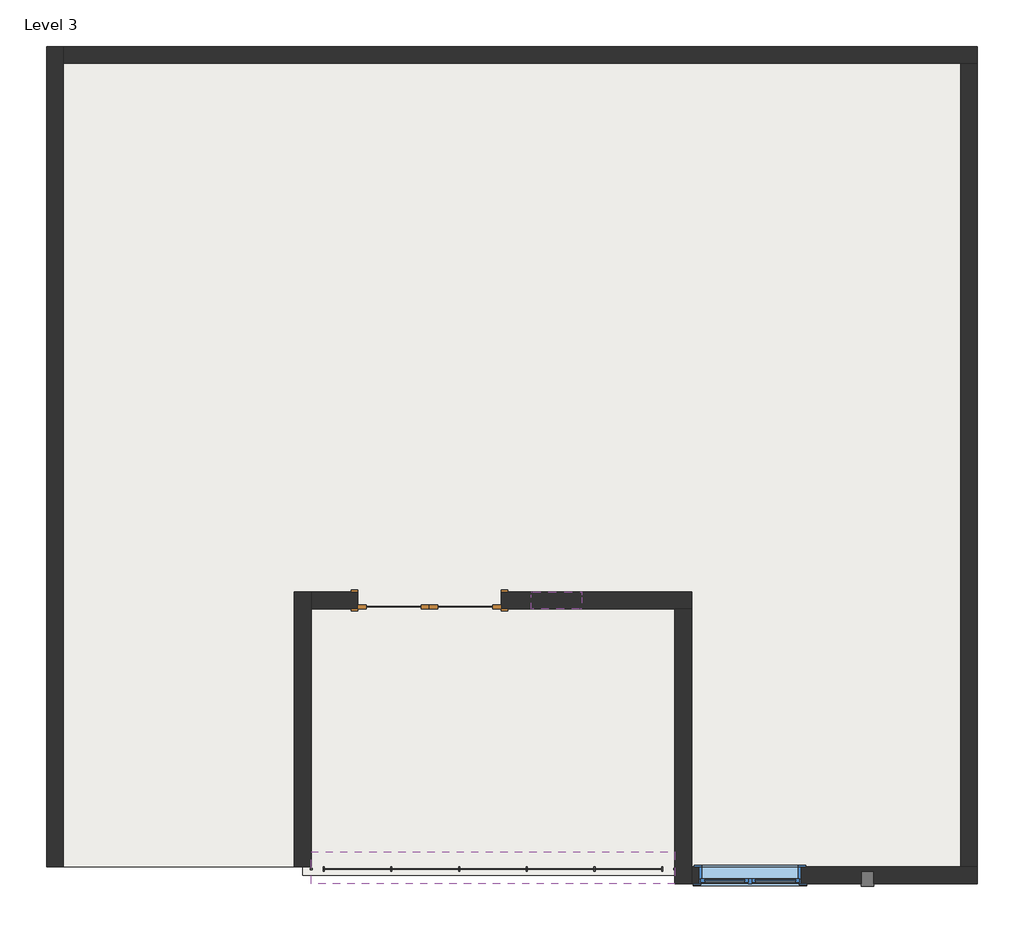
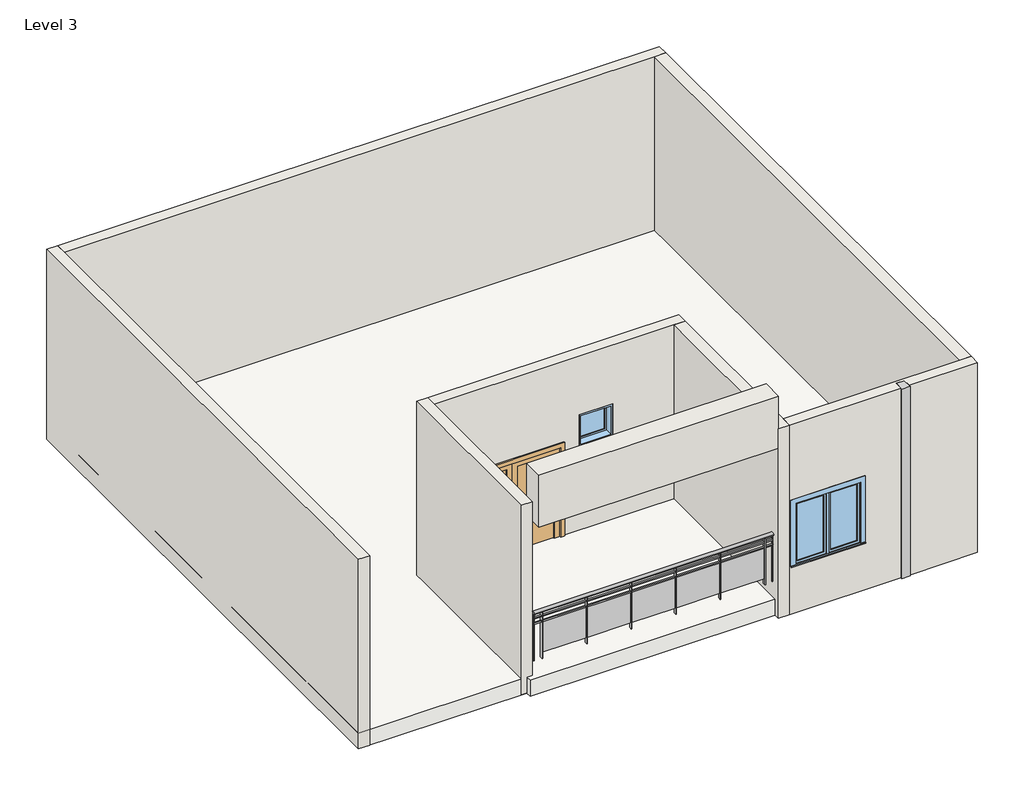
# One storey: 8 walls, 2 windows, 1 door, 1 proxy, 1 railing, 1 roof.
"""IFC4 building model written with IfcOpenShell, lengths in millimetres."""

from ifc_helpers import new_model, si_unit, point, frame, origin, place, context, project, spatial, polyline, ellipse_curve, trimmed, outline, extrude, faceted_brep, transform, mapped, element, save
from ifc_brep_helpers import plane_surface, extruded_surface, advanced_brep
from components import door_10418eaf, walls_2_walls_2_a0716ef0, window_0862ab64, window_6846e476

model = new_model("IFC4")

# Units and contexts
model_context = context("Model", 3, world=origin())
ifc_project = project(units=[si_unit("LENGTHUNIT", "METRE", prefix="MILLI")], contexts=[model_context])

# Site, building, storey
site = spatial("IfcSite", under=ifc_project)
building = spatial("IfcBuilding", under=site)
storey = spatial("IfcBuildingStorey", under=building, Name="Level 3", Elevation=7315.2)

# Proxy
placement = place(None, origin())
element("IfcBuildingElementProxy", 1, Name="Reveal", ObjectType="Reveal", at=placement, inside=storey, context=model_context, shape_type="SweptSolid", body=[
    extrude(outline(polyline([(752.5001186, 242.2810824), (752.5001186, 425.1610824), (904.9001186, 425.1610824), (904.9001186, 242.2810824), (752.5001186, 242.2810824)])), frame((0.0, 0.0, 7315.2), z_axis=(0.0, 0.0, 1.0), x_axis=(1.0, 0.0, 0.0)), (0.0, 0.0, 1.0), 3657.6),
])

# Door
door_shape = door_10418eaf(model_context)
element("IfcDoor", 2, ObjectType="Door-Double-Glass : 68\" x 80\"", at=placement, inside=storey, context=model_context, shape_type="MappedRepresentation", body=[
    mapped(door_shape, transform((-4429.0998814, 3678.7423324, 7315.2), x_axis=(-1.0, 0.0, 0.0), y_axis=(0.0, -1.0, 0.0), z_axis=(0.0, 0.0, 1.0))),
])

# Railing
element("IfcRailing", 3, ObjectType="Glass Panel - Bottom Fill", at=placement, inside=storey, context=model_context, shape_type="SolidModel", body=[
    advanced_brep(
    [(-5851.4998814, 488.6610824, 8839.2), (-5851.4998814, 412.4610824, 8839.2), (-1482.6998814, 488.6610824, 8839.2), (-1482.6998814, 412.4610824, 8839.2)],
    [
        (0, 1, ellipse_curve(frame((-5851.4998814, 450.5610824, 8839.2), z_axis=(-1.0, 0.0, 0.0), x_axis=(0.0, -1.0, 0.0)), 38.1, 28.575)),
        (1, 0, ellipse_curve(frame((-5851.4998814, 450.5610824, 8839.2), z_axis=(-1.0, 0.0, 0.0), x_axis=(0.0, -1.0, 0.0)), 38.1, 28.575)),
        (2, 3, ellipse_curve(frame((-1482.6998814, 450.5610824, 8839.2), z_axis=(1.0, 0.0, 0.0), x_axis=(0.0, -1.0, 0.0)), 38.1, 28.575)),
        (3, 2, ellipse_curve(frame((-1482.6998814, 450.5610824, 8839.2), z_axis=(1.0, 0.0, 0.0), x_axis=(0.0, -1.0, 0.0)), 38.1, 28.575)),
        (0, 2),
        (3, 1),
    ],
    [
        plane_surface(frame((-5851.4998814, 450.5610824, 8839.2), z_axis=(-1.0, 0.0, 0.0), x_axis=(0.0, 1.0, 0.0))),
        plane_surface(frame((-1482.6998814, 450.5610824, 8839.2), z_axis=(1.0, 0.0, 0.0), x_axis=(0.0, 1.0, 0.0))),
        extruded_surface(trimmed(ellipse_curve(frame((-1482.6998814, 450.5610824, 8839.2), z_axis=(-1.0, 0.0, 0.0), x_axis=(0.0, -1.0, 0.0)), 38.1, 28.575), [point((-1482.6998814, 488.6610824, 8839.2))], [point((-1482.6998814, 412.4610824, 8839.2))], True, "CARTESIAN"), (-4368.8, 0.0, 0.0), 4368.8),
        extruded_surface(trimmed(ellipse_curve(frame((-1482.6998814, 450.5610824, 8839.2), z_axis=(-1.0, 0.0, 0.0), x_axis=(0.0, -1.0, 0.0)), 38.1, 28.575), [point((-1482.6998814, 412.4610824, 8839.2))], [point((-1482.6998814, 488.6610824, 8839.2))], True, "CARTESIAN"), (-4368.8, 0.0, 0.0), 4368.8),
    ],
    [
        (0, [[1, 2]]),
        (1, [[3, 4]]),
        (2, [[-1, 5, -4, 6]]),
        (3, [[-2, -6, -3, -5]]),
    ],
),
    extrude(outline(polyline([(-5851.4998814, 437.8610824), (-5851.4998814, 463.2610824), (-1482.6998814, 463.2610824), (-1482.6998814, 437.8610824), (-5851.4998814, 437.8610824)])), frame((0.0, 0.0, 8724.9), z_axis=(0.0, 0.0, 1.0), x_axis=(1.0, 0.0, 0.0)), (0.0, 0.0, 1.0), 25.4),
    extrude(outline(polyline([(-5851.4998814, 437.8610824), (-5851.4998814, 463.2610824), (-1482.6998814, 463.2610824), (-1482.6998814, 437.8610824), (-5851.4998814, 437.8610824)])), frame((0.0, 0.0, 8623.3), z_axis=(0.0, 0.0, 1.0), x_axis=(1.0, 0.0, 0.0)), (0.0, 0.0, 1.0), 25.4),
    extrude(outline(polyline([(-1641.4498814, 425.1610824), (-1641.4498814, 475.9610824), (-1628.7498814, 475.9610824), (-1628.7498814, 425.1610824), (-1641.4498814, 425.1610824)])), frame((0.0, 0.0, 7924.8), z_axis=(0.0, 0.0, 1.0), x_axis=(1.0, 0.0, 0.0)), (0.0, 0.0, 1.0), 885.6788223),
    extrude(outline(polyline([(-2447.8998814, 457.0962394), (-1635.0998814, 457.0962394), (-1635.0998814, 450.7462394), (-2447.8998814, 450.7462394), (-2447.8998814, 457.0962394)])), frame((0.0, 0.0, 8026.4), z_axis=(0.0, 0.0, 1.0), x_axis=(1.0, 0.0, 0.0)), (0.0, 0.0, 1.0), 596.9),
    extrude(outline(polyline([(-2454.2498814, 425.1610824), (-2454.2498814, 475.9610824), (-2441.5498814, 475.9610824), (-2441.5498814, 425.1610824), (-2454.2498814, 425.1610824)])), frame((0.0, 0.0, 7924.8), z_axis=(0.0, 0.0, 1.0), x_axis=(1.0, 0.0, 0.0)), (0.0, 0.0, 1.0), 885.6788223),
    extrude(outline(polyline([(-3260.6998814, 457.0962394), (-2447.8998814, 457.0962394), (-2447.8998814, 450.7462394), (-3260.6998814, 450.7462394), (-3260.6998814, 457.0962394)])), frame((0.0, 0.0, 8026.4), z_axis=(0.0, 0.0, 1.0), x_axis=(1.0, 0.0, 0.0)), (0.0, 0.0, 1.0), 596.9),
    extrude(outline(polyline([(-3267.0498814, 425.1610824), (-3267.0498814, 475.9610824), (-3254.3498814, 475.9610824), (-3254.3498814, 425.1610824), (-3267.0498814, 425.1610824)])), frame((0.0, 0.0, 7924.8), z_axis=(0.0, 0.0, 1.0), x_axis=(1.0, 0.0, 0.0)), (0.0, 0.0, 1.0), 885.6788223),
    extrude(outline(polyline([(-4073.4998814, 457.0962394), (-3260.6998814, 457.0962394), (-3260.6998814, 450.7462394), (-4073.4998814, 450.7462394), (-4073.4998814, 457.0962394)])), frame((0.0, 0.0, 8026.4), z_axis=(0.0, 0.0, 1.0), x_axis=(1.0, 0.0, 0.0)), (0.0, 0.0, 1.0), 596.9),
    extrude(outline(polyline([(-4079.8498814, 425.1610824), (-4079.8498814, 475.9610824), (-4067.1498814, 475.9610824), (-4067.1498814, 425.1610824), (-4079.8498814, 425.1610824)])), frame((0.0, 0.0, 7924.8), z_axis=(0.0, 0.0, 1.0), x_axis=(1.0, 0.0, 0.0)), (0.0, 0.0, 1.0), 885.6788223),
    extrude(outline(polyline([(-4886.2998814, 457.0962394), (-4073.4998814, 457.0962394), (-4073.4998814, 450.7462394), (-4886.2998814, 450.7462394), (-4886.2998814, 457.0962394)])), frame((0.0, 0.0, 8026.4), z_axis=(0.0, 0.0, 1.0), x_axis=(1.0, 0.0, 0.0)), (0.0, 0.0, 1.0), 596.9),
    extrude(outline(polyline([(-4892.6498814, 425.1610824), (-4892.6498814, 475.9610824), (-4879.9498814, 475.9610824), (-4879.9498814, 425.1610824), (-4892.6498814, 425.1610824)])), frame((0.0, 0.0, 7924.8), z_axis=(0.0, 0.0, 1.0), x_axis=(1.0, 0.0, 0.0)), (0.0, 0.0, 1.0), 885.6788223),
    extrude(outline(polyline([(-5699.0998814, 457.0962394), (-4886.2998814, 457.0962394), (-4886.2998814, 450.7462394), (-5699.0998814, 450.7462394), (-5699.0998814, 457.0962394)])), frame((0.0, 0.0, 8026.4), z_axis=(0.0, 0.0, 1.0), x_axis=(1.0, 0.0, 0.0)), (0.0, 0.0, 1.0), 596.9),
    extrude(outline(polyline([(-5705.4498814, 425.1610824), (-5705.4498814, 475.9610824), (-5692.7498814, 475.9610824), (-5692.7498814, 425.1610824), (-5705.4498814, 425.1610824)])), frame((0.0, 0.0, 7924.8), z_axis=(0.0, 0.0, 1.0), x_axis=(1.0, 0.0, 0.0)), (0.0, 0.0, 1.0), 885.6788223),
    extrude(outline(polyline([(-1495.3998814, 441.0360824), (-1495.3998814, 460.0860824), (-1476.3498814, 460.0860824), (-1476.3498814, 441.0360824), (-1495.3998814, 441.0360824)])), frame((0.0, 0.0, 7924.8), z_axis=(0.0, 0.0, 1.0), x_axis=(1.0, 0.0, 0.0)), (0.0, 0.0, 1.0), 885.6788223),
    extrude(outline(polyline([(-5857.8498814, 441.0360824), (-5857.8498814, 460.0860824), (-5838.7998814, 460.0860824), (-5838.7998814, 441.0360824), (-5857.8498814, 441.0360824)])), frame((0.0, 0.0, 7924.8), z_axis=(0.0, 0.0, 1.0), x_axis=(1.0, 0.0, 0.0)), (0.0, 0.0, 1.0), 885.6788223),
])

# Roof
element("IfcRoof", 4, ObjectType="Generic - 12\"", at=placement, inside=storey, context=model_context, shape_type="SweptSolid", body=[
    extrude(outline(polyline([(-9026.4998814, 10331.1610824), (2149.5001186, 10331.1610824), (2149.5001186, 374.3610824), (-5953.0998814, 374.3610824), (-5953.0998814, 475.9610824), (-9026.4998814, 475.9610824), (-9026.4998814, 10331.1610824)])), frame((0.0, 0.0, 7315.2), z_axis=(0.0, 0.0, 1.0), x_axis=(1.0, 0.0, 0.0)), (0.0, 0.0, 1.0), 304.8),
])

# Walls
element("IfcWall", 5, ObjectType="Generic - 8\"", at=placement, inside=storey, context=model_context, shape_type="Brep", body=[
    faceted_brep([(-5851.4998814, 475.9610824, 7315.2), (-5851.4998814, 3574.7610824, 7315.2), (-5851.4998814, 3777.9610824, 7315.2), (-5851.4998814, 3777.9610824, 10972.8), (-5851.4998814, 3574.7610824, 10972.8), (-5851.4998814, 475.9610824, 10972.8), (-6054.6998814, 475.9610824, 7315.2), (-6054.6998814, 475.9610824, 10972.8), (-6054.6998814, 3777.9610824, 10972.8), (-6054.6998814, 3777.9610824, 7315.2)], [[[0, 1, 2, 3, 4, 5]], [[6, 7, 8, 9]], [[2, 1, 0, 6, 9]], [[5, 4, 3, 8, 7]], [[0, 5, 7, 6]], [[3, 2, 9, 8]]]),
])
element("IfcWall", 6, ObjectType="Generic - 8\"", at=placement, inside=storey, context=model_context, shape_type="Brep", body=[
    faceted_brep([(-5851.4998814, 3574.7610824, 7315.2), (-5292.6998814, 3574.7610824, 7315.2), (-5292.6998814, 3574.7610824, 9347.2), (-3565.4998814, 3574.7610824, 9347.2), (-3565.4998814, 3574.7610824, 7315.2), (-1482.6998814, 3574.7610824, 7315.2), (-1279.4998814, 3574.7610824, 7315.2), (-1279.4998814, 3574.7610824, 10972.8), (-1482.6998814, 3574.7610824, 10972.8), (-5851.4998814, 3574.7610824, 10972.8), (-2600.2998814, 3574.7610824, 9842.1899962), (-2600.2998814, 3574.7610824, 9232.5899962), (-3209.8998814, 3574.7610824, 9232.5899962), (-3209.8998814, 3574.7610824, 9842.1899962), (-5292.6998814, 3777.9610824, 9347.2), (-5292.6998814, 3777.9610824, 7315.2), (-5851.4998814, 3777.9610824, 7315.2), (-5851.4998814, 3777.9610824, 10972.8), (-1279.4998814, 3777.9610824, 10972.8), (-1279.4998814, 3777.9610824, 7315.2), (-3565.4998814, 3777.9610824, 7315.2), (-3565.4998814, 3777.9610824, 9347.2), (-2600.2998814, 3777.9610824, 9842.1899962), (-3209.8998814, 3777.9610824, 9842.1899962), (-3209.8998814, 3777.9610824, 9232.5899962), (-2600.2998814, 3777.9610824, 9232.5899962)], [[[0, 1, 2, 3, 4, 5, 6, 7, 8, 9], [10, 11, 12, 13]], [[14, 15, 16, 17, 18, 19, 20, 21], [22, 23, 24, 25]], [[20, 19, 6, 5, 4]], [[16, 15, 1, 0]], [[9, 8, 7, 18, 17]], [[0, 9, 17, 16]], [[7, 6, 19, 18]], [[11, 10, 22, 25]], [[12, 11, 25, 24]], [[13, 12, 24, 23]], [[10, 13, 23, 22]], [[2, 1, 15, 14]], [[3, 2, 14, 21]], [[4, 3, 21, 20]]]),
])
element("IfcWall", 7, ObjectType="Generic - 8\"", at=placement, inside=storey, context=model_context, shape_type="Brep", body=[
    faceted_brep([(-1482.6998814, 3574.7610824, 7315.2), (-1482.6998814, 272.7610824, 7315.2), (-1482.6998814, 272.7610824, 10972.8), (-1482.6998814, 3574.7610824, 10972.8), (-1279.4998814, 3574.7610824, 7315.2), (-1279.4998814, 3574.7610824, 10972.8), (-1279.4998814, 475.9610824, 10972.8), (-1279.4998814, 272.7610824, 10972.8), (-1279.4998814, 272.7610824, 7315.2), (-1279.4998814, 475.9610824, 7315.2)], [[[0, 1, 2, 3]], [[4, 5, 6, 7, 8, 9]], [[1, 0, 4, 9, 8]], [[3, 2, 7, 6, 5]], [[0, 3, 5, 4]], [[2, 1, 8, 7]]]),
])
element("IfcWall", 8, ObjectType="Generic - 8\"", at=placement, inside=storey, context=model_context, shape_type="Brep", body=[
    faceted_brep([(-1279.4998814, 272.7610824, 10972.8), (-1279.4998814, 272.7610824, 7315.2), (752.5001186, 272.7610824, 7315.2), (752.5001186, 272.7610824, 10972.8), (-1190.5998814, 272.7610824, 8229.6), (-1190.5998814, 272.7610824, 9448.8), (28.6001186, 272.7610824, 9448.8), (28.6001186, 272.7610824, 8229.6), (2149.5001186, 272.7610824, 7315.2), (2149.5001186, 272.7610824, 10972.8), (904.9001186, 272.7610824, 10972.8), (904.9001186, 272.7610824, 7315.2), (2149.5001186, 475.9610824, 7315.2), (1946.3001186, 475.9610824, 7315.2), (-1279.4998814, 475.9610824, 7315.2), (-1279.4998814, 475.9610824, 10972.8), (1946.3001186, 475.9610824, 10972.8), (2149.5001186, 475.9610824, 10972.8), (-1190.5998814, 475.9610824, 9448.8), (-1190.5998814, 475.9610824, 8229.6), (28.6001186, 475.9610824, 8229.6), (28.6001186, 475.9610824, 9448.8), (904.9001186, 425.1610824, 7315.2), (752.5001186, 425.1610824, 7315.2), (752.5001186, 425.1610824, 10972.8), (904.9001186, 425.1610824, 10972.8)], [[[0, 1, 2, 3], [4, 5, 6, 7]], [[8, 9, 10, 11]], [[12, 13, 14, 15, 16, 17], [18, 19, 20, 21]], [[14, 13, 12, 8, 11, 22, 23, 2, 1]], [[17, 16, 15, 0, 3, 24, 25, 10, 9]], [[1, 0, 15, 14]], [[9, 8, 12, 17]], [[19, 18, 5, 4]], [[20, 19, 4, 7]], [[21, 20, 7, 6]], [[18, 21, 6, 5]], [[25, 22, 11, 10]], [[22, 25, 24, 23]], [[23, 24, 3, 2]]]),
])
element("IfcWall", 9, ObjectType="Generic - 8\"", at=placement, inside=storey, context=model_context, shape_type="Brep", body=[
    faceted_brep([(-8823.2998814, 475.9610824, 7315.2), (-8823.2998814, 10127.9610824, 7315.2), (-8823.2998814, 10331.1610824, 7315.2), (-8823.2998814, 10331.1610824, 10972.8), (-8823.2998814, 10127.9610824, 10972.8), (-8823.2998814, 475.9610824, 10972.8), (-9026.4998814, 475.9610824, 7315.2), (-9026.4998814, 475.9610824, 10972.8), (-9026.4998814, 10331.1610824, 10972.8), (-9026.4998814, 10331.1610824, 7315.2)], [[[0, 1, 2, 3, 4, 5]], [[6, 7, 8, 9]], [[2, 1, 0, 6, 9]], [[5, 4, 3, 8, 7]], [[0, 5, 7, 6]], [[3, 2, 9, 8]]]),
])
element("IfcWall", 10, ObjectType="Generic - 8\"", at=placement, inside=storey, context=model_context, shape_type="Brep", body=[
    faceted_brep([(-8823.2998814, 10127.9610824, 7315.2), (1946.3001186, 10127.9610824, 7315.2), (2149.5001186, 10127.9610824, 7315.2), (2149.5001186, 10127.9610824, 10972.8), (1946.3001186, 10127.9610824, 10972.8), (-8823.2998814, 10127.9610824, 10972.8), (-8823.2998814, 10331.1610824, 7315.2), (-8823.2998814, 10331.1610824, 10972.8), (2149.5001186, 10331.1610824, 10972.8), (2149.5001186, 10331.1610824, 7315.2)], [[[0, 1, 2, 3, 4, 5]], [[6, 7, 8, 9]], [[2, 1, 0, 6, 9]], [[5, 4, 3, 8, 7]], [[0, 5, 7, 6]], [[3, 2, 9, 8]]]),
])
element("IfcWall", 11, ObjectType="Generic - 8\"", at=placement, inside=storey, context=model_context, shape_type="SweptSolid", body=[
    extrude(outline(polyline([(1946.3001186, 475.9610824), (1946.3001186, 10127.9610824), (2149.5001186, 10127.9610824), (2149.5001186, 475.9610824), (1946.3001186, 475.9610824)])), frame((0.0, 0.0, 7315.2), z_axis=(0.0, 0.0, 1.0), x_axis=(1.0, 0.0, 0.0)), (0.0, 0.0, 1.0), 3657.6),
])
walls_2_walls_2_shape = walls_2_walls_2_a0716ef0(model_context)
element("IfcWall", 12, ObjectType="Walls 2 : Walls 2", at=placement, inside=storey, context=model_context, shape_type="MappedRepresentation", body=[
    mapped(walls_2_walls_2_shape, transform((0.0, 0.0, 0.0), x_axis=(1.0, 0.0, 0.0), y_axis=(0.0, 1.0, 0.0), z_axis=(0.0, 0.0, 1.0))),
])

# Windows
window_shape = window_0862ab64(model_context)
element("IfcWindow", 13, ObjectType="Casement Dbl with Trim.0001 : 48\" x 48\"", at=placement, inside=storey, context=model_context, shape_type="MappedRepresentation", body=[
    mapped(window_shape, transform((-580.9998814, 393.4110824, 7315.2), x_axis=(-1.0, 0.0, 0.0), y_axis=(0.0, -1.0, 0.0), z_axis=(0.0, 0.0, 1.0))),
])
window_2_shape = window_6846e476(model_context)
element("IfcWindow", 14, ObjectType="Fixed : 24\" x 24\"", at=placement, inside=storey, context=model_context, shape_type="MappedRepresentation", body=[
    mapped(window_2_shape, transform((-2866.9998814, 3676.3610824, 8318.1899962), x_axis=(1.0, 0.0, 0.0), y_axis=(0.0, 1.0, 0.0), z_axis=(0.0, 0.0, 1.0))),
])

save(model, "model.ifc")

# Revit data of these elements
# Type "Door-Double-Glass : 68\" x 80\""
#   Type Mark = "8"
#   Construction Type Id = "opn-d45"
#   Assembly Code = "C1020"
#   Analytic Construction = "Wood frame, double glass door "
#   W = 2' - 10"
#   Thickness = 0' - 2"
#   Thermal Resistance (R) = 1.8150 (h·ft²·°F)/BTU
#   Swing Angle [instance default] = 90.00°
#   Heat Transfer Coefficient (U) = 0.5510 BTU/(h·ft²·°F)
#   Height = 6' - 8"
#   Bottom Rail = 0' - 4"
#   Top Rail = 0' - 4"
#   Stiles = 0' - 4"
#   Trim Projection = 0' - 1"
#   Trim Width = 0' - 3"
#   Width = 5' - 8"
#   Define Thermal Properties by = 1
#   Glazing = Glass
#   Panel Material = Wood - Birch - Solid Stained Light Low Gloss
#   Trim Material = Paint - Sienna
#   Visual Light Transmittance = 0
#   Solar Heat Gain Coefficient = 0
#   Function = (empty or 0)
#   Wall Closure = (empty or 0)
# Type "Glass Panel - Bottom Fill"
#   Assembly Code = "C2010400"
#   built-in parameter 1008612 = 0.0416667 (stored number, unit not read)
#   built-in parameter 1008611 = 0.0416667 (stored number, unit not read)
#   built-in parameter 1008609 = 0.333333 (stored number, unit not read)
#   built-in parameter 1008604 = 0.166667 (stored number, unit not read)
#   built-in parameter 1008603 = 0.166667 (stored number, unit not read)
#   Railing Height = 3' - 0"
#   built-in parameter 1008630 = 2
#   built-in parameter 1008610 = 2
#   built-in parameter 1008618 = Baluster - Square : 3/4"
# Type "Generic - 12\""
#   Assembly Code = "B1020"
#   Layers, outside or top first: 1' - 0" no material (function 1)
# Type "Generic - 8\""
#   Assembly Code = "B2010"
#   Layers, outside or top first: 0' - 8" no material (function 1)
# Type "Casement Dbl with Trim.0001 : 48\" x 48\""
#   Type Mark = "14"
#   Construction Type Id = "GSP4R"
#   Assembly Code = "B2020100"
#   Analytic Construction = "1/8 in Pilkington single glazing"
#   Visual Light Transmittance = 0.9
#   Solar Heat Gain Coefficient = 0.78
#   Heat Transfer Coefficient (U) = 0.6496 BTU/(h·ft²·°F)
#   Height = 4' - 0"
#   Default Sill Height = 3' - 0"
#   Trim Projection - Ext. = 0' - 0 1/2"
#   Trim Projection - Int. = 0' - 0 3/4"
#   Trim Width - Exterior = 0' - 3 1/2"
#   Trim Width - Interior = 0' - 3 1/2"
#   Width = 4' - 0"
#   Window Inset = 0' - 0 3/4"
#   Define Thermal Properties by = 1
#   Glass Pane Material = Glass
#   Sash Material = Sash
#   Trim Exterior Material = Trim
#   Trim Interior Material = Trim
#   Wall Closure = (empty or 0)
# Type "Fixed : 24\" x 24\""
#   Type Mark = "3"
#   Construction Type Id = "GSP4R"
#   Assembly Code = "B2020100"
#   Analytic Construction = "1/8 in Pilkington single glazing"
#   Visual Light Transmittance = 0.9
#   Solar Heat Gain Coefficient = 0.78
#   Heat Transfer Coefficient (U) = 0.6496 BTU/(h·ft²·°F)
#   Height = 2' - 0"
#   Default Sill Height = 3' - 0"
#   Width = 2' - 0"
#   Window Inset = 0' - 0 3/4"
#   Define Thermal Properties by = 1
#   Glass Pane Material = Glass
#   Sash Material = Sash
#   Wall Closure = (empty or 0)
# Element 2 (IfcDoor, "Door-Double-Glass : 68\" x 80\"")
#   Swing Angle = 90.00°
#   Phase Created = New Construction
#   Materials on its faces: "Wood - Birch - Solid Stained Light Low Gloss", "Paint - Sienna", "Glass"
# Element 3 (IfcRailing, "Glass Panel - Bottom Fill")
#   built-in parameter 1008621 = 2 (stored number, unit not read)
#   Phase Created = New Construction
#   Materials on its faces: "Glass"
# Element 4 (IfcRoof, "Generic - 12\"")
#   built-in parameter 1001705 = 25 (stored number, unit not read)
#   built-in parameter 1001710 = 33615
#   Phase Created = New Construction
#   Materials on its faces: "Default Roof"
# Elements 5, 6, 7, 8, 9, 10, 11 (IfcWall, "Generic - 8\"")
#   Top Offset = 0' - 0"
#   Base Offset = 0' - 0"
#   Unconnected Height = 12' - 0"
#   wall height = 12' - 0"
#   Phase Created = New Construction
#   Base Constraint = Level 3
#   Materials on its faces: "Default Wall"
# Element 12 (IfcWall, "Walls 2 : Walls 2")
#   Phase Created = New Construction
#   Materials on its faces: "Default Wall"
# Element 13 (IfcWindow, "Casement Dbl with Trim.0001 : 48\" x 48\"")
#   Mark = "4"
#   Phase Created = New Construction
#   Materials on its faces: "Sash", "Trim", "Glass"
# Element 14 (IfcWindow, "Fixed : 24\" x 24\"")
#   Mark = "7"
#   Phase Created = New Construction
#   Materials on its faces: "Sash", "Glass"
# Materials
#   "Glass": class "Glass", colour RGB 0 128 192, transparency 0.75, Description = "Soda Lime Glass", Cost = 0
#   "Wood - Birch - Solid Stained Light Low Gloss": class "Wood", colour RGB 210 159 95, transparency 0, Cost = 0
#   "Paint - Sienna": colour RGB 118 70 51, transparency 0, Cost = 0
#   "Sash": class "Wood", colour RGB 224 178 126, transparency 0
#   "Trim": class "Wood", colour RGB 224 178 126, transparency 0
#   "Default Roof": colour RGB 88 101 114, transparency 0
#   "Default Wall": colour RGB 128 128 128, transparency 0
